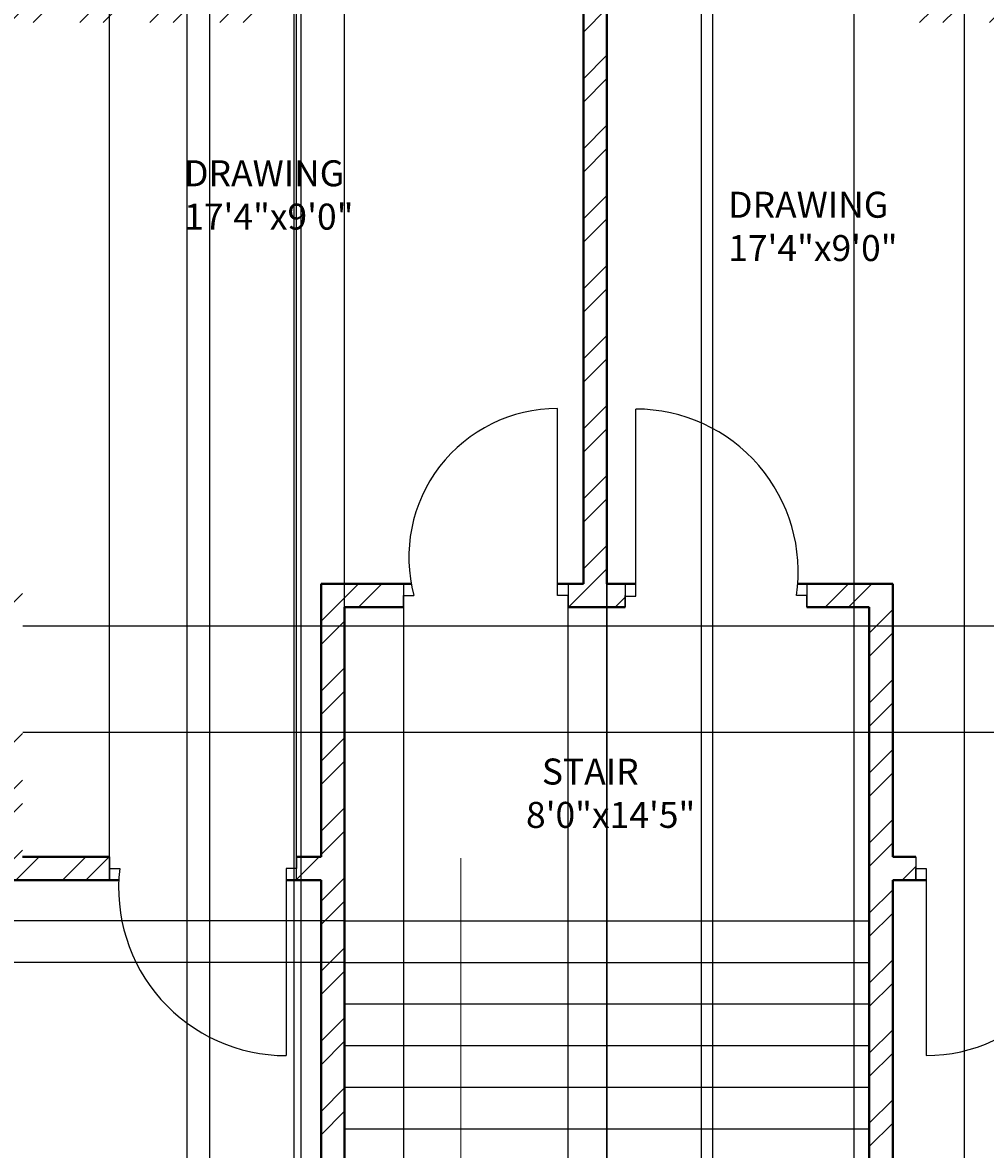
# Model space of a CAD drawing. Units: inches. Extents: x 2063 to 2617, y 1299 to 2210.
# Tile 3 of 22: x 2228 to 2414, y 1510 to 1727. Entities that reach past the tile are written whole.
import ezdxf

# ---------------------------------------------------------------- set-up
doc = ezdxf.new("R2010")
doc.units = ezdxf.units.IN
for name, color, linetype, lineweight in [('A-ANNO-DIMS', 2, 'Continuous', 18), ('A-ANNO-SYMB', 171, 'Continuous', 18), ('A-AREA-IDEN', 7, 'Continuous', 18), ('A-DOOR', 11, 'Continuous', 25), ('A-FLOR-STRS', 171, 'Continuous', 25), ('A-WALL', 7, 'Continuous', 40)]:
    doc.layers.add(name, color=color, linetype=linetype, lineweight=lineweight)
doc.layers.add('A-WALL-PATT', color=215, linetype='Continuous', lineweight=13, true_color=0xa953a0)
doc.styles.get("Standard").update_dxf_attribs({"font": 'arial.ttf'})
doc.dimstyles.get("Standard").update_dxf_attribs({"dimtxt": 0.18, "dimasz": 0.18, "dimexe": 0.18, "dimexo": 0.0625, "dimgap": 0.09, "dimtad": 0, "dimtih": 1, "dimtoh": 1, "dimdec": 4, "dimzin": 0, "dimdsep": 46, "dimtxsty": 'Standard', "dimcen": 0.09, "dimadec": 0, "dimazin": 0, "dimtfac": 1, "dimtdec": 4, "dimtofl": 0, "dimtmove": 0, "dimatfit": 3, "dimfxl": 1, "dimtolj": 1, "dimtzin": 0, "dimarcsym": 0})

# ---------------------------------------------------------------- blocks, each defined once
blk = doc.blocks.new('*D50')
at = {"layer": 'A-ANNO-DIMS', "color": 0, "lineweight": -2, "transparency": 16777216}
for p, q in [((2264.14, 2124.25), (2264.14, 1317.7)), ((2280.35, 2124.25), (2280.35, 1317.7)), ((2264.32, 1317.88), (2271.79, 1317.88)), ((2280.17, 1317.88), (2272.7, 1317.88))]:
    blk.add_line(p, q, dxfattribs=at)
at = {"layer": 'A-ANNO-DIMS', "color": 0, "transparency": 16777216}
for points in [[(2264.32, 1317.91), (2264.32, 1317.85), (2264.14, 1317.88)], [(2280.17, 1317.91), (2280.17, 1317.85), (2280.35, 1317.88)]]:
    blk.add_solid(points, dxfattribs=at)
at = {"layer": 'Defpoints', "color": 0, "transparency": 16777216}
for p in [(2264.14, 2124.31), (2280.35, 2124.31), (2280.35, 1317.88)]:
    blk.add_point(p, dxfattribs=at)
at = {"layer": 'A-ANNO-DIMS', "color": 0, "transparency": 16777216, "insert": (2272.25, 1317.88), "char_height": 0.18, "attachment_point": 5}
blk.add_mtext('\\A1;16.204', dxfattribs=at)
blk = doc.blocks.new('*D51')
at = {"layer": 'A-ANNO-DIMS', "color": 0, "lineweight": -2, "transparency": 16777216}
for p, q in [((2340.64, 2124.25), (2340.64, 1317.7)), ((2358.75, 2124.25), (2358.75, 1317.7)), ((2340.82, 1317.88), (2349.24, 1317.88)), ((2358.57, 1317.88), (2350.15, 1317.88))]:
    blk.add_line(p, q, dxfattribs=at)
at = {"layer": 'A-ANNO-DIMS', "color": 0, "transparency": 16777216}
for points in [[(2340.82, 1317.91), (2340.82, 1317.85), (2340.64, 1317.88)], [(2358.57, 1317.91), (2358.57, 1317.85), (2358.75, 1317.88)]]:
    blk.add_solid(points, dxfattribs=at)
at = {"layer": 'Defpoints', "color": 0, "transparency": 16777216}
for p in [(2340.64, 2124.31), (2358.75, 2124.31), (2358.75, 1317.88)]:
    blk.add_point(p, dxfattribs=at)
at = {"layer": 'A-ANNO-DIMS', "color": 0, "transparency": 16777216, "insert": (2349.7, 1317.88), "char_height": 0.18, "attachment_point": 5}
blk.add_mtext('\\A1;18.106', dxfattribs=at)
blk = doc.blocks.new('*D54')
at = {"layer": 'A-ANNO-DIMS', "color": 0, "lineweight": -2, "transparency": 16777216}
for p, q in [((2340.64, 2124.25), (2340.64, 1317.7)), ((2360.96, 2104.46), (2360.96, 1317.7)), ((2340.82, 1317.88), (2350.34, 1317.88)), ((2360.78, 1317.88), (2351.27, 1317.88))]:
    blk.add_line(p, q, dxfattribs=at)
at = {"layer": 'A-ANNO-DIMS', "color": 0, "transparency": 16777216}
for points in [[(2340.82, 1317.91), (2340.82, 1317.85), (2340.64, 1317.88)], [(2360.78, 1317.91), (2360.78, 1317.85), (2360.96, 1317.88)]]:
    blk.add_solid(points, dxfattribs=at)
at = {"layer": 'Defpoints', "color": 0, "transparency": 16777216}
for p in [(2340.64, 2124.31), (2360.96, 2104.52), (2360.96, 1317.88)]:
    blk.add_point(p, dxfattribs=at)
at = {"layer": 'A-ANNO-DIMS', "color": 0, "transparency": 16777216, "insert": (2350.8, 1317.88), "char_height": 0.18, "attachment_point": 5}
blk.add_mtext('\\A1;20.317', dxfattribs=at)
blk = doc.blocks.new('*D55')
at = {"layer": 'A-ANNO-DIMS', "color": 0, "lineweight": -2, "transparency": 16777216}
for p, q in [((2388.15, 1975.75), (2388.15, 1317.7)), ((2409.37, 1975.75), (2409.37, 1317.7)), ((2388.33, 1317.88), (2398.3, 1317.88)), ((2409.19, 1317.88), (2399.23, 1317.88))]:
    blk.add_line(p, q, dxfattribs=at)
at = {"layer": 'A-ANNO-DIMS', "color": 0, "transparency": 16777216}
for points in [[(2388.33, 1317.91), (2388.33, 1317.85), (2388.15, 1317.88)], [(2409.19, 1317.91), (2409.19, 1317.85), (2409.37, 1317.88)]]:
    blk.add_solid(points, dxfattribs=at)
at = {"layer": 'Defpoints', "color": 0, "transparency": 16777216}
for p in [(2388.15, 1975.81), (2409.37, 1975.81), (2409.37, 1317.88)]:
    blk.add_point(p, dxfattribs=at)
at = {"layer": 'A-ANNO-DIMS', "color": 0, "transparency": 16777216, "insert": (2398.76, 1317.88), "char_height": 0.18, "attachment_point": 5}
blk.add_mtext('\\A1;21.225', dxfattribs=at)
blk = doc.blocks.new('*D58')
at = {"layer": 'A-ANNO-DIMS', "color": 0, "lineweight": -2, "transparency": 16777216}
for p, q in [((2290.08, 1554.5), (2081.21, 1554.5)), ((2081.39, 1554.32), (2081.39, 1550.68)), ((2081.39, 1546.68), (2081.39, 1550.32)), ((2290.08, 1546.5), (2081.21, 1546.5))]:
    blk.add_line(p, q, dxfattribs=at)
at = {"layer": 'A-ANNO-DIMS', "color": 0, "transparency": 16777216}
for points in [[(2081.36, 1554.32), (2081.42, 1554.32), (2081.39, 1554.5)], [(2081.36, 1546.68), (2081.42, 1546.68), (2081.39, 1546.5)]]:
    blk.add_solid(points, dxfattribs=at)
at = {"layer": 'Defpoints', "color": 0, "transparency": 16777216}
for p in [(2081.39, 1554.5), (2290.14, 1554.5), (2290.14, 1546.5)]:
    blk.add_point(p, dxfattribs=at)
at = {"layer": 'A-ANNO-DIMS', "color": 0, "transparency": 16777216, "insert": (2081.39, 1550.5), "char_height": 0.18, "attachment_point": 5}
blk.add_mtext('\\A1;8', dxfattribs=at)
blk = doc.blocks.new('*D59')
at = {"layer": 'A-ANNO-DIMS', "color": 0, "lineweight": -2, "transparency": 16777216}
for p, q in [((2290.14, 1554.56), (2290.14, 2170.74)), ((2290.32, 2170.56), (2315.07, 2170.56)), ((2340.46, 2170.56), (2315.72, 2170.56)), ((2340.64, 1554.56), (2340.64, 2170.74))]:
    blk.add_line(p, q, dxfattribs=at)
at = {"layer": 'A-ANNO-DIMS', "color": 0, "transparency": 16777216}
for points in [[(2290.32, 2170.59), (2290.32, 2170.53), (2290.14, 2170.56)], [(2340.46, 2170.59), (2340.46, 2170.53), (2340.64, 2170.56)]]:
    blk.add_solid(points, dxfattribs=at)
at = {"layer": 'Defpoints', "color": 0, "transparency": 16777216}
for p in [(2340.64, 2170.56), (2290.14, 1554.5), (2340.64, 1554.5)]:
    blk.add_point(p, dxfattribs=at)
at = {"layer": 'A-ANNO-DIMS', "color": 0, "transparency": 16777216, "insert": (2315.39, 2170.56), "char_height": 0.18, "attachment_point": 5}
blk.add_mtext('\\A1;50.5', dxfattribs=at)
blk = doc.blocks.new('*D60')
at = {"layer": 'A-ANNO-DIMS', "color": 0, "lineweight": -2, "transparency": 16777216}
for p, q in [((2301.46, 1614.75), (2301.46, 1317.7)), ((2333.14, 1614.75), (2333.14, 1317.7)), ((2301.64, 1317.88), (2316.84, 1317.88)), ((2332.96, 1317.88), (2317.76, 1317.88))]:
    blk.add_line(p, q, dxfattribs=at)
at = {"layer": 'A-ANNO-DIMS', "color": 0, "transparency": 16777216}
for points in [[(2301.64, 1317.91), (2301.64, 1317.85), (2301.46, 1317.88)], [(2332.96, 1317.91), (2332.96, 1317.85), (2333.14, 1317.88)]]:
    blk.add_solid(points, dxfattribs=at)
at = {"layer": 'Defpoints', "color": 0, "transparency": 16777216}
for p in [(2301.46, 1614.81), (2333.14, 1614.81), (2333.14, 1317.88)]:
    blk.add_point(p, dxfattribs=at)
at = {"layer": 'A-ANNO-DIMS', "color": 0, "transparency": 16777216, "insert": (2317.3, 1317.88), "char_height": 0.18, "attachment_point": 5}
blk.add_mtext('\\A1;31.684', dxfattribs=at)
blk = doc.blocks.new('*D62')
at = {"layer": 'A-ANNO-DIMS', "color": 0, "lineweight": -2, "transparency": 16777216}
for p, q in [((2259.81, 1437.87), (2259.81, 2170.74)), ((2259.99, 2170.56), (2270.4, 2170.56)), ((2281.61, 2170.56), (2271.19, 2170.56)), ((2281.79, 1437.87), (2281.79, 2170.74))]:
    blk.add_line(p, q, dxfattribs=at)
at = {"layer": 'A-ANNO-DIMS', "color": 0, "transparency": 16777216}
for points in [[(2259.99, 2170.59), (2259.99, 2170.53), (2259.81, 2170.56)], [(2281.61, 2170.59), (2281.61, 2170.53), (2281.79, 2170.56)]]:
    blk.add_solid(points, dxfattribs=at)
at = {"layer": 'Defpoints', "color": 0, "transparency": 16777216}
for p in [(2281.79, 2170.56), (2259.81, 1437.81), (2281.79, 1437.81)]:
    blk.add_point(p, dxfattribs=at)
at = {"layer": 'A-ANNO-DIMS', "color": 0, "transparency": 16777216, "insert": (2270.8, 2170.56), "char_height": 0.18, "attachment_point": 5}
blk.add_mtext('\\A1;21.98', dxfattribs=at)
blk = doc.blocks.new('*D63')
at = {"layer": 'A-ANNO-DIMS', "color": 0, "lineweight": -2, "transparency": 16777216}
for p, q in [((2244.87, 1562.37), (2244.87, 2170.74)), ((2245.05, 2170.56), (2262.4, 2170.56)), ((2280.68, 2170.56), (2263.33, 2170.56)), ((2280.86, 1562.37), (2280.86, 2170.74))]:
    blk.add_line(p, q, dxfattribs=at)
at = {"layer": 'A-ANNO-DIMS', "color": 0, "transparency": 16777216}
for points in [[(2245.05, 2170.59), (2245.05, 2170.53), (2244.87, 2170.56)], [(2280.68, 2170.59), (2280.68, 2170.53), (2280.86, 2170.56)]]:
    blk.add_solid(points, dxfattribs=at)
at = {"layer": 'Defpoints', "color": 0, "transparency": 16777216}
for p in [(2280.86, 2170.56), (2244.87, 1562.31), (2280.86, 1562.31)]:
    blk.add_point(p, dxfattribs=at)
at = {"layer": 'A-ANNO-DIMS', "color": 0, "transparency": 16777216, "insert": (2262.86, 2170.56), "char_height": 0.18, "attachment_point": 5}
blk.add_mtext('\\A1;35.995', dxfattribs=at)
blk = doc.blocks.new('*D68')
at = {"layer": 'A-ANNO-DIMS', "color": 0, "lineweight": -2, "transparency": 16777216}
for p, q in [((2228.21, 1611.27), (2595.57, 1611.27)), ((2595.39, 1611.09), (2595.39, 1601.22)), ((2595.39, 1590.99), (2595.39, 1600.86)), ((2228.21, 1590.81), (2595.57, 1590.81))]:
    blk.add_line(p, q, dxfattribs=at)
at = {"layer": 'A-ANNO-DIMS', "color": 0, "transparency": 16777216}
for points in [[(2595.36, 1611.09), (2595.42, 1611.09), (2595.39, 1611.27)], [(2595.36, 1590.99), (2595.42, 1590.99), (2595.39, 1590.81)]]:
    blk.add_solid(points, dxfattribs=at)
at = {"layer": 'Defpoints', "color": 0, "transparency": 16777216}
for p in [(2228.14, 1611.27), (2595.39, 1611.27), (2228.14, 1590.81)]:
    blk.add_point(p, dxfattribs=at)
at = {"layer": 'A-ANNO-DIMS', "color": 0, "transparency": 16777216, "insert": (2595.39, 1601.04), "char_height": 0.18, "attachment_point": 5}
blk.add_mtext('\\A1;20.46', dxfattribs=at)

msp = doc.modelspace()

# ---------------------------------------------------------------- hatches: boundary and pattern name
at = {"layer": 'A-WALL-PATT'}
h = msp.add_hatch(dxfattribs=at)
h.set_pattern_fill('ANSI32', color=256)
h.paths.add_polyline_path([(2553.6442, 2128.8122), (2511.1703, 2128.8122), (2511.1703, 2124.3122), (2549.1442, 2124.3122), (2549.1442, 2095.662), (2553.6442, 2095.662)])
h.paths.add_polyline_path([(2553.6442, 2035.662), (2549.1442, 2035.662), (2549.1442, 1980.3122), (2503.7214, 1980.3122), (2503.7214, 1975.8122), (2549.1442, 1975.8122), (2549.1442, 1962.9693), (2553.6442, 1962.9693)])
h.paths.add_polyline_path([(2553.6442, 1938.9693), (2549.1442, 1938.9693), (2549.1442, 1927.8122), (2477.1442, 1927.8122), (2477.1442, 1975.8122), (2481.2918, 1975.8122), (2481.2918, 1980.3122), (2453.2648, 1980.3122), (2453.2648, 1975.8122), (2472.6442, 1975.8122), (2472.6442, 1868.3122), (2400.6442, 1868.3122), (2400.6442, 1861.3782), (2405.1442, 1861.3782), (2405.1442, 1863.8122), (2480.9699, 1863.8122), (2480.9699, 1866.0622), (2480.9699, 1868.3122), (2477.1442, 1868.3122), (2477.1442, 1923.3122), (2549.1442, 1923.3122), (2549.1442, 1908.8504), (2553.6442, 1908.8504)])
h.paths.add_polyline_path([(2553.6442, 1884.8504), (2549.1442, 1884.8504), (2549.1442, 1868.3122), (2501.0636, 1868.3122), (2501.0636, 1863.8122), (2549.1442, 1863.8122), (2549.1442, 1826.0298), (2553.6442, 1826.0298)])
h.paths.add_polyline_path([(2388.1504, 1980.3122), (2340.6442, 1980.3122), (2340.6442, 2124.3122), (2358.7501, 2124.3122), (2358.7501, 2128.8122), (2316.3482, 2128.8122), (2316.3482, 2124.3122), (2336.1442, 2124.3122), (2336.1442, 1980.3122), (2289.1737, 1980.3122), (2289.1737, 1975.8122), (2336.1442, 1975.8122), (2336.1442, 1619.3122), (2333.1433, 1619.3122), (2333.1433, 1614.8122), (2344.1671, 1614.8122), (2344.1671, 1617.0622), (2344.1671, 1619.3122), (2340.6442, 1619.3122), (2340.6442, 1975.8122), (2388.1504, 1975.8122), (2388.1504, 1978.0622)])
h.paths.add_polyline_path([(2290.1442, 1614.8122), (2301.4594, 1614.8122), (2301.4594, 1617.0622), (2301.4594, 1619.3122), (2285.6442, 1619.3122), (2285.6442, 1566.8122), (2280.8619, 1566.8122), (2280.8619, 1564.5622), (2280.8619, 1562.3122), (2285.6442, 1562.3122), (2285.6442, 1442.3122), (2281.7879, 1442.3122), (2281.7879, 1437.8122), (2285.6442, 1437.8122), (2285.6442, 1401.8122), (2290.1442, 1401.8122)])
h.paths.add_polyline_path([(2549.1442, 1731.8122), (2405.1442, 1731.8122), (2405.1442, 1834.4638), (2402.8942, 1834.4638), (2400.6442, 1834.4638), (2400.6442, 1727.3122), (2549.1442, 1727.3122)])
h.paths.add_polyline_path([(2553.6442, 1766.0298), (2551.3942, 1766.0298), (2549.1442, 1766.0298), (2549.1442, 1686.7767), (2553.6442, 1686.7767)])
h.paths.add_polyline_path([(2553.6442, 1638.7767), (2551.3942, 1638.7767), (2549.1442, 1638.7767), (2549.1442, 1619.3122), (2448.6442, 1619.3122), (2448.6442, 1610.5671), (2450.8942, 1610.5671), (2453.1442, 1610.5671), (2453.1442, 1614.8122), (2549.1442, 1614.8122), (2549.1442, 1601.6421), (2553.6442, 1601.6421)])
h.paths.add_polyline_path([(2553.6442, 1577.6421), (2551.3942, 1577.6421), (2549.1442, 1577.6421), (2549.1442, 1566.8122), (2453.1442, 1566.8122), (2453.1442, 1591.5045), (2451.0335, 1591.5045), (2448.6442, 1591.5045), (2448.6442, 1566.8122), (2434.0475, 1566.8122), (2434.0475, 1562.3122), (2549.1442, 1562.3122), (2549.1442, 1533.48), (2553.6442, 1533.48)])
h.paths.add_polyline_path([(2553.6442, 1473.48), (2549.1442, 1473.48), (2549.1442, 1442.3122), (2502.6258, 1442.3122), (2502.6258, 1437.8122), (2549.1442, 1437.8122), (2549.1442, 1401.8122), (2553.6442, 1401.8122)])
h.paths.add_polyline_path([(2395.6442, 1562.3122), (2400.0901, 1562.3122), (2400.0901, 1564.5622), (2400.0901, 1566.8122), (2395.6442, 1566.8122), (2395.6442, 1619.3122), (2379.1127, 1619.3122), (2379.1127, 1614.8122), (2391.1442, 1614.8122), (2391.1442, 1401.8122), (2395.6442, 1401.8122), (2395.6442, 1437.8122), (2399.2425, 1437.8122), (2399.2425, 1440.0622), (2399.2425, 1442.3122), (2395.6442, 1442.3122)])
h.paths.add_polyline_path([(2442.6258, 1442.3122), (2419.6262, 1442.3122), (2419.6262, 1437.8122), (2442.6258, 1437.8122), (2442.6258, 1440.0622)])
h.paths.add_polyline_path([(2127.6442, 1480.2532), (2125.3942, 1480.2532), (2123.1442, 1480.2532), (2123.1442, 1401.8122), (2127.6442, 1401.8122), (2127.6442, 1437.8122), (2145.1538, 1437.8122), (2145.1538, 1440.0622), (2145.1538, 1442.3122), (2127.6442, 1442.3122)])
h.paths.add_polyline_path([(2259.809, 1442.3122), (2205.1538, 1442.3122), (2205.1538, 1437.8122), (2259.809, 1437.8122), (2259.809, 1440.0622)])
h.paths.add_polyline_path([(2127.6442, 1659.7652), (2123.1442, 1659.7652), (2123.1442, 1605.5161), (2125.3942, 1605.5161), (2127.6442, 1605.5161), (2127.6442, 1614.8122), (2223.6442, 1614.8122), (2223.6442, 1611.2723), (2228.1442, 1611.2723), (2228.1442, 1619.3122), (2127.6442, 1619.3122)])
h.paths.add_polyline_path([(2244.8673, 1566.8122), (2228.1442, 1566.8122), (2228.1442, 1590.8122), (2225.8942, 1590.8122), (2223.6442, 1590.8122), (2223.6442, 1566.8122), (2127.6442, 1566.8122), (2127.6442, 1581.5161), (2123.1442, 1581.5161), (2123.1442, 1540.2532), (2127.6442, 1540.2532), (2127.6442, 1562.3122), (2244.8673, 1562.3122), (2244.8673, 1564.5622)])
h.paths.add_polyline_path([(2172.5174, 1868.3122), (2127.6442, 1868.3122), (2127.6442, 1886.5833), (2123.1442, 1886.5833), (2123.1442, 1832.6633), (2127.6442, 1832.6633), (2127.6442, 1863.8122), (2172.5174, 1863.8122), (2172.5174, 1866.0622)])
h.paths.add_polyline_path([(2276.1442, 1868.3122), (2204.1442, 1868.3122), (2204.1442, 1923.3122), (2204.1442, 1975.8122), (2224.8362, 1975.8122), (2224.8362, 1978.1097), (2224.8362, 1980.3122), (2195.0729, 1980.3122), (2195.0729, 1978.0622), (2195.0729, 1975.8122), (2199.6442, 1975.8122), (2199.6442, 1927.8122), (2127.6442, 1927.8122), (2127.6442, 1942.3492), (2123.1442, 1942.3492), (2123.1442, 1910.5833), (2127.6442, 1910.5833), (2127.6442, 1923.3122), (2199.6442, 1923.3122), (2199.6442, 1868.3122), (2194.8228, 1868.3122), (2194.8228, 1864.7337), (2194.8228, 1863.8122), (2271.6442, 1863.8122), (2271.6442, 1860.0507), (2276.1442, 1860.0507)])
h.paths.add_polyline_path([(2276.1442, 1829.994), (2273.8942, 1829.994), (2271.6442, 1829.994), (2271.6442, 1731.8122), (2127.6442, 1731.8122), (2127.6442, 1772.6633), (2123.1442, 1772.6633), (2123.1442, 1707.7652), (2127.6442, 1707.7652), (2127.6442, 1727.3122), (2276.1442, 1727.3122)])
h.paths.add_polyline_path([(2127.6442, 2022.1152), (2123.1442, 2022.1152), (2123.1442, 1966.3492), (2127.6442, 1966.3492), (2127.6442, 1975.8122), (2174.2082, 1975.8122), (2174.2082, 1978.0622), (2174.2082, 1980.3122), (2127.6442, 1980.3122)])
h.paths.add_polyline_path([(2361.9755, 1678.588), (2398.4558, 1678.588), (2398.4558, 1697.2453), (2361.9755, 1697.2453)], flags=9)
h.paths.add_polyline_path([(2351.5397, 1780.4072), (2386.1987, 1780.4072), (2386.1987, 1790.7107), (2351.5397, 1790.7107)], flags=25)
h.paths.add_polyline_path([(2350.6753, 1940.9321), (2387.6024, 1940.9321), (2387.6024, 1959.5894), (2350.6753, 1959.5894)], flags=25)
h.paths.add_polyline_path([(2254.9545, 1684.638), (2295.0943, 1684.638), (2295.0943, 1703.2953), (2254.9545, 1703.2953)], flags=9)
h.paths.add_polyline_path([(2282.4946, 1782.4438), (2317.1535, 1782.4438), (2317.1535, 1792.7474), (2282.4946, 1792.7474)], flags=9)
h.paths.add_polyline_path([(2270.327, 1939.2854), (2307.254, 1939.2854), (2307.254, 1957.9428), (2270.327, 1957.9428)], flags=9)

# ---------------------------------------------------------------- linework, layer by layer
at = {"layer": 'A-ANNO-SYMB'}
msp.add_line((2312.4997, 1566.5449), (2312.4997, 1421.896), dxfattribs=at)
at = {"layer": 'A-DOOR'}
for p, q in [((2331.1433, 1617.0622), (2331.1433, 1653.0622)), ((2346.1671, 1616.9445), (2346.1671, 1652.9445)), ((2301.4594, 1619.3122), (2301.4594, 1614.8122)), ((2333.1433, 1619.3122), (2333.1433, 1614.8122)), ((2344.1671, 1619.3122), (2344.1671, 1614.8122)), ((2379.1127, 1619.3122), (2379.1127, 1614.8122)), ((2301.4594, 1614.8122), (2301.4594, 1617.0622)), ((2301.4594, 1617.0622), (2303.4594, 1617.0622)), ((2333.1433, 1617.0622), (2331.1433, 1617.0622)), ((2333.1433, 1614.8122), (2333.1433, 1617.0622)), ((2344.1671, 1614.8122), (2344.1671, 1617.0622)), ((2344.1671, 1617.0622), (2344.1671, 1616.9445)), ((2344.1671, 1616.9445), (2346.1671, 1616.9445)), ((2379.1127, 1617.0622), (2377.1127, 1617.0622)), ((2379.1127, 1614.8122), (2379.1127, 1617.0622)), ((2244.8673, 1566.8122), (2244.8673, 1562.3122)), ((2280.8619, 1562.3122), (2280.8619, 1566.8122)), ((2280.8619, 1566.8122), (2280.8619, 1564.5622)), ((2400.0901, 1566.8122), (2400.0901, 1562.3122)), ((2244.8673, 1562.3122), (2244.8673, 1564.5622)), ((2244.8673, 1564.5622), (2246.8673, 1564.5622)), ((2280.8619, 1564.5622), (2278.8619, 1564.5622)), ((2278.8619, 1564.5622), (2278.8619, 1528.5622)), ((2400.0901, 1562.3122), (2400.0901, 1564.5622)), ((2400.0901, 1564.5622), (2402.0901, 1564.5622)), ((2402.0901, 1564.5622), (2402.0901, 1528.5622))]:
    msp.add_line(p, q, dxfattribs=at)
for centre, radius, start, end in [((2331.1433, 1624.4178), 28.6444, 90, 194.879685), ((2346.1671, 1621.6593), 31.2852, 351.550271, 90), ((2278.8619, 1560.7796), 32.2175, 173.257561, 270), ((2402.0901, 1559.0267), 30.4645, 270, 10.468944)]:
    msp.add_arc(centre, radius, start, end, dxfattribs=at)
at = {"layer": 'A-FLOR-STRS'}
for p, q in [((2290.1442, 1554.4994), (2391.1442, 1554.4994)), ((2340.6442, 1434.4994), (2340.6442, 1554.4994)), ((2290.1442, 1546.4994), (2391.1442, 1546.4994)), ((2290.1442, 1538.4994), (2391.1442, 1538.4994)), ((2290.1442, 1530.4994), (2391.1442, 1530.4994)), ((2290.1442, 1522.4994), (2391.1442, 1522.4994)), ((2290.1442, 1514.4994), (2391.1442, 1514.4994))]:
    msp.add_line(p, q, dxfattribs=at)
at = {"layer": 'A-WALL'}
for p, q in [((2336.1442, 1975.8122), (2336.1442, 1619.3122)), ((2340.6442, 1975.8122), (2340.6442, 1619.3122)), ((2285.6442, 1619.3122), (2285.6442, 1566.8122)), ((2302.9576, 1619.3122), (2285.6442, 1619.3122)), ((2336.1442, 1619.3122), (2331.1433, 1619.3122)), ((2346.1671, 1619.3122), (2340.6442, 1619.3122)), ((2395.6442, 1619.3122), (2377.3642, 1619.3122)), ((2395.6442, 1619.3122), (2395.6442, 1566.8122)), ((2290.1442, 1614.8122), (2290.1442, 1401.8122)), ((2301.4594, 1614.8122), (2290.1442, 1614.8122)), ((2344.1671, 1614.8122), (2333.1433, 1614.8122)), ((2391.1442, 1614.8122), (2379.1127, 1614.8122)), ((2391.1442, 1614.8122), (2391.1442, 1401.8122)), ((2228.1442, 1566.8122), (2244.8673, 1566.8122)), ((2280.8619, 1566.8122), (2285.6442, 1566.8122)), ((2395.6442, 1566.8122), (2400.0901, 1566.8122)), ((2127.6442, 1562.3122), (2246.6809, 1562.3122)), ((2278.8619, 1562.3122), (2285.6442, 1562.3122)), ((2285.6442, 1562.3122), (2285.6442, 1442.3122)), ((2395.6442, 1562.3122), (2402.0901, 1562.3122)), ((2395.6442, 1562.3122), (2395.6442, 1442.3122))]:
    msp.add_line(p, q, dxfattribs=at)

# ---------------------------------------------------------------- texts
at = {"layer": 'A-AREA-IDEN', "char_height": 5, "attachment_point": 1}
for s, width, insert in [('  DRAWING\\P  17\'4"x9\'0"', 109.322466, (2256.2045, 1700.8072)), ('DRAWING\\P17\'4"x9\'0"', 142.579183, (2363.9861, 1694.7573)), ('      STAIR\\P    8\'0"x14\'5" ', 113.103459, (2318.9441, 1585.7065))]:
    msp.add_mtext_dynamic_manual_height_columns(s, width=width, gutter_width=12.5, heights=[0], dxfattribs=dict(at, insert=insert))

# ---------------------------------------------------------------- dimensions: what is measured, and where the dimension line sits
at = {"layer": 'A-ANNO-DIMS'}
for base, p1, p2, override, picture, middle in [((2280.8619, 2170.5622), (2244.8673, 1562.3122), (2280.8619, 1562.3122), {"dimdec": 3, "dimlfac": 1, "dimrnd": 0, "dimzin": 0, "dimdsep": 46, "dimlunit": 2}, '*D63', (2262.8646, 2170.5622)), ((2281.7879, 2170.5622), (2259.809, 1437.8122), (2281.7879, 1437.8122), {"dimdec": 2, "dimlfac": 1, "dimrnd": 0, "dimzin": 0, "dimdsep": 46, "dimlunit": 2}, '*D62', (2270.7984, 2170.5622)), ((2340.6442, 2170.5622), (2290.1442, 1554.4994), (2340.6442, 1554.4994), {"dimdec": 1, "dimlfac": 1, "dimrnd": 0, "dimzin": 0, "dimdsep": 46, "dimlunit": 2}, '*D59', (2315.3942, 2170.5622)), ((2280.3482, 1317.8821), (2264.1442, 2124.3122), (2280.3482, 2124.3122), {"dimdec": 3, "dimlfac": 1, "dimrnd": 0, "dimzin": 0, "dimdsep": 46, "dimlunit": 2}, '*D50', (2272.2462, 1317.8821)), ((2358.7501, 1317.8821), (2340.6442, 2124.3122), (2358.7501, 2124.3122), {"dimdec": 3, "dimlfac": 1, "dimrnd": 0, "dimzin": 0, "dimdsep": 46, "dimlunit": 2}, '*D51', (2349.6972, 1317.8821)), ((2360.9612, 1317.8821), (2340.6442, 2124.3122), (2360.9612, 2104.5201), {"dimdec": 3, "dimlfac": 1, "dimrnd": 0, "dimzin": 0, "dimdsep": 46, "dimlunit": 2}, '*D54', (2350.8027, 1317.8821)), ((2409.375, 1317.8821), (2388.1504, 1975.8122), (2409.375, 1975.8122), {"dimdec": 3, "dimlfac": 1, "dimrnd": 0, "dimzin": 0, "dimdsep": 46, "dimlunit": 2}, '*D55', (2398.7627, 1317.8821)), ((2333.1433, 1317.8821), (2301.4594, 1614.8122), (2333.1433, 1614.8122), {"dimdec": 3, "dimlfac": 1, "dimrnd": 0, "dimzin": 0, "dimdsep": 46, "dimlunit": 2}, '*D60', (2317.3014, 1317.8821))]:
    dim = msp.add_linear_dim(base=base, p1=p1, p2=p2, dimstyle='Standard', override=override, dxfattribs=at)
    dim.commit()
    dim.dimension.update_dxf_attribs({"geometry": picture, "text_midpoint": middle})
for base, p1, p2, override, picture, middle in [((2595.3943, 1611.2723), (2228.1442, 1590.8122), (2228.1442, 1611.2723), {"dimdec": 2, "dimlfac": 1, "dimrnd": 0, "dimzin": 0, "dimdsep": 46, "dimlunit": 2}, '*D68', (2595.3943, 1601.0422)), ((2081.3943, 1554.4994), (2290.1442, 1546.4994), (2290.1442, 1554.4994), {"dimdec": 0, "dimlfac": 1, "dimrnd": 0, "dimzin": 0, "dimdsep": 46, "dimlunit": 2}, '*D58', (2081.3943, 1550.4994))]:
    dim = msp.add_linear_dim(base=base, p1=p1, p2=p2, angle=90, dimstyle='Standard', override=override, dxfattribs=at)
    dim.commit()
    dim.dimension.update_dxf_attribs({"geometry": picture, "text_midpoint": middle})

doc.saveas('drawing.dxf')
